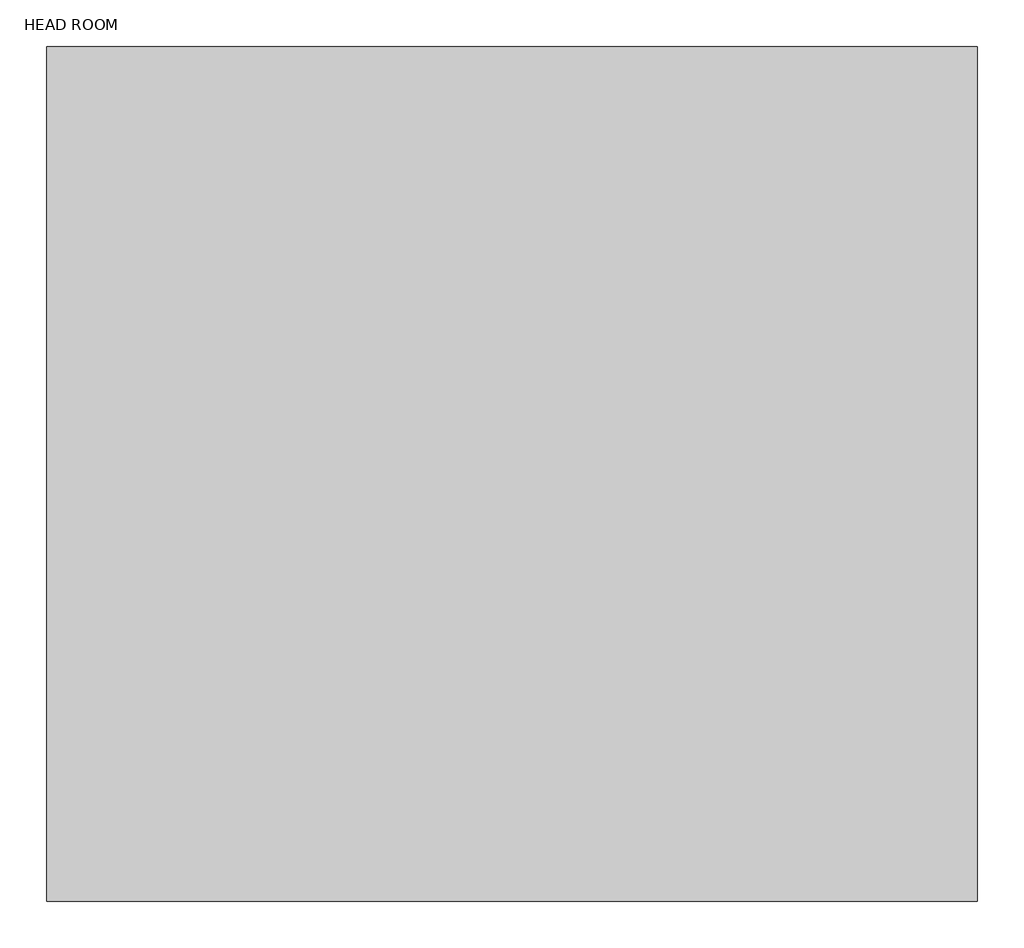
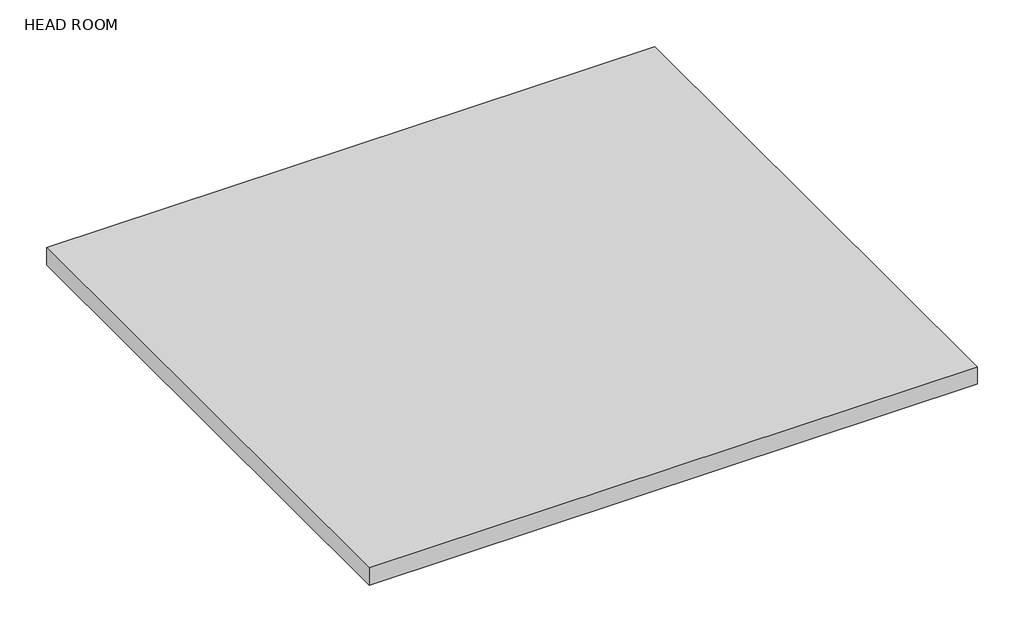
# One storey: 1 proxy.
"""IFC4 building model written with IfcOpenShell, lengths in millimetres."""

from ifc_helpers import new_model, si_unit, origin, place, context, project, spatial, transform, mapped, element, save
from components import generic_models_1_generic_models_1_ab7b9371

model = new_model("IFC4")

# Units and contexts
model_context = context("Model", 3, world=origin())
ifc_project = project(units=[si_unit("LENGTHUNIT", "METRE", prefix="MILLI")], contexts=[model_context])

# Site, building, storey
site = spatial("IfcSite", under=ifc_project)
building = spatial("IfcBuilding", under=site)
storey = spatial("IfcBuildingStorey", under=building, Name="HEAD ROOM", Elevation=9448.8)

# Proxy
placement = place(None, origin())
generic_models_1_generic_models_1_shape = generic_models_1_generic_models_1_ab7b9371(model_context)
element("IfcBuildingElementProxy", 1, Name="Generic Models 1 : Generic Models 1", ObjectType="Generic Models 1 : Generic Models 1", at=placement, inside=storey, context=model_context, shape_type="MappedRepresentation", body=[
    mapped(generic_models_1_generic_models_1_shape, transform((0.0, 0.0, 0.0), x_axis=(1.0, 0.0, 0.0), y_axis=(0.0, 1.0, 0.0), z_axis=(0.0, 0.0, 1.0))),
])

save(model, "model.ifc")

# Revit data of these elements
# Element 1 (IfcBuildingElementProxy, "Generic Models 1 : Generic Models 1")
#   Phase Created = New Construction
#   Materials on its faces: "Clad - White"
# Materials
#   "Clad - White": class "Wood", colour RGB 242 242 238, transparency 0, Cost = 0
